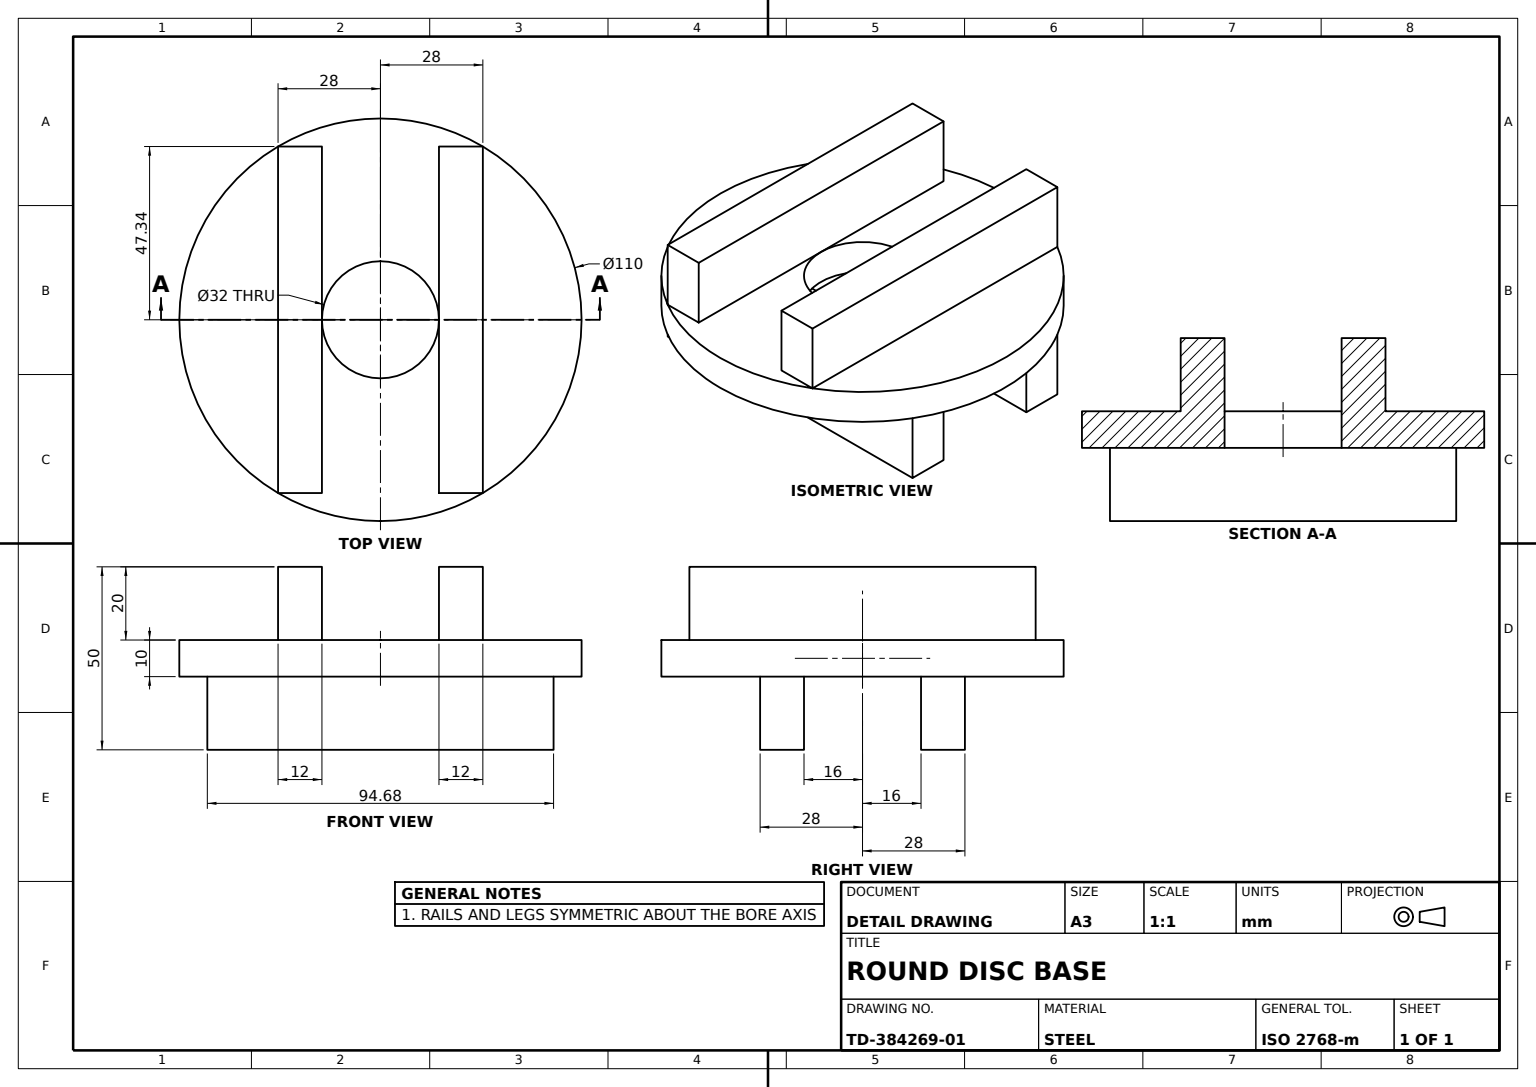
SolidWorks part; units mm, degrees
material "Plain Carbon Steel"
ref_plane "Front Plane" through (0, 0, 0) normal (0, 0, 1) x (1, 0, 0)
ref_plane "Top Plane" through (0, 0, 0) normal (0, 1, 0) x (1, 0, 0)
ref_plane "Right Plane" through (0, 0, 0) normal (1, 0, 0) x (0, 0, -1)
sketch "Base Disc Sketch" plane through (0, 0, 0) normal (0, 1, 0) x (1, 0, 0)
  circle A0 centre (0, 0) radius 55
  circle A1 centre (0, 0) radius 16
  dimension "D1" = 110
  dimension "D2" = 32
extrude "Base Disc Ø110 Bore Ø32" add sketch "Base Disc Sketch" along normal blind 10
sketch "Top Rails Sketch" plane through (0, 10, 0) normal (0, 1, 0) x (1, 0, 0)
  line L0 (28, -47.3392) -> (28, 47.3392)
  line L2 (-16, -47.3392) -> (-28, -47.3392)
  line L3 (-16, -47.3392) -> (-16, 47.3392)
  line L4 (-16, 47.3392) -> (-28, 47.3392)
  line L5 (-28, -47.3392) -> (-28, 47.3392)
  line L6 (16, 47.3392) -> (28, 47.3392)
  line L7 (16, -47.3392) -> (16, 47.3392)
  line L8 (16, -47.3392) -> (28, -47.3392)
  circle A2 centre (0, 0) radius 55 construction
  dimension "D1" = 16
  dimension "D2" = 28
  dimension "D3" = 16
  dimension "D4" = 47.3392
extrude "Top Rails" add sketch "Top Rails Sketch" along normal blind 20
sketch "Bottom Legs Sketch" plane through (0, 0, 0) normal (0, -1, 0) x (1, 0, 0)
  line L0 (-83.9759, 0) -> (90.7824, 0)
  line L2 (47.3392, -16) -> (47.3392, -28)
  line L3 (47.3392, -16) -> (-47.3392, -16)
  line L4 (-47.3392, -16) -> (-47.3392, -28)
  line L5 (47.3392, -28) -> (-47.3392, -28)
  line L10 (47.3392, 28) -> (-47.3392, 28)
  line L11 (-47.3392, 16) -> (-47.3392, 28)
  line L12 (47.3392, 16) -> (-47.3392, 16)
  line L13 (47.3392, 16) -> (47.3392, 28)
  circle A1 centre (0, 0) radius 55 construction
  point P8 (0, -22)
  point P22 (0, 22)
  dimension "D1" = 94.6784
  dimension "D2" = 12
  dimension "D3" = 16
  dimension "D4" = 22
  dimension "D5" = 22
  dimension "D6" = 83.9759
  dimension "D7" = 90.7824
  dimension "D8" = 47.3392
extrude "Bottom Legs" add sketch "Bottom Legs Sketch" along normal blind 20 contours L12 L13 L10 L11 | L5 L2 L3 L4
